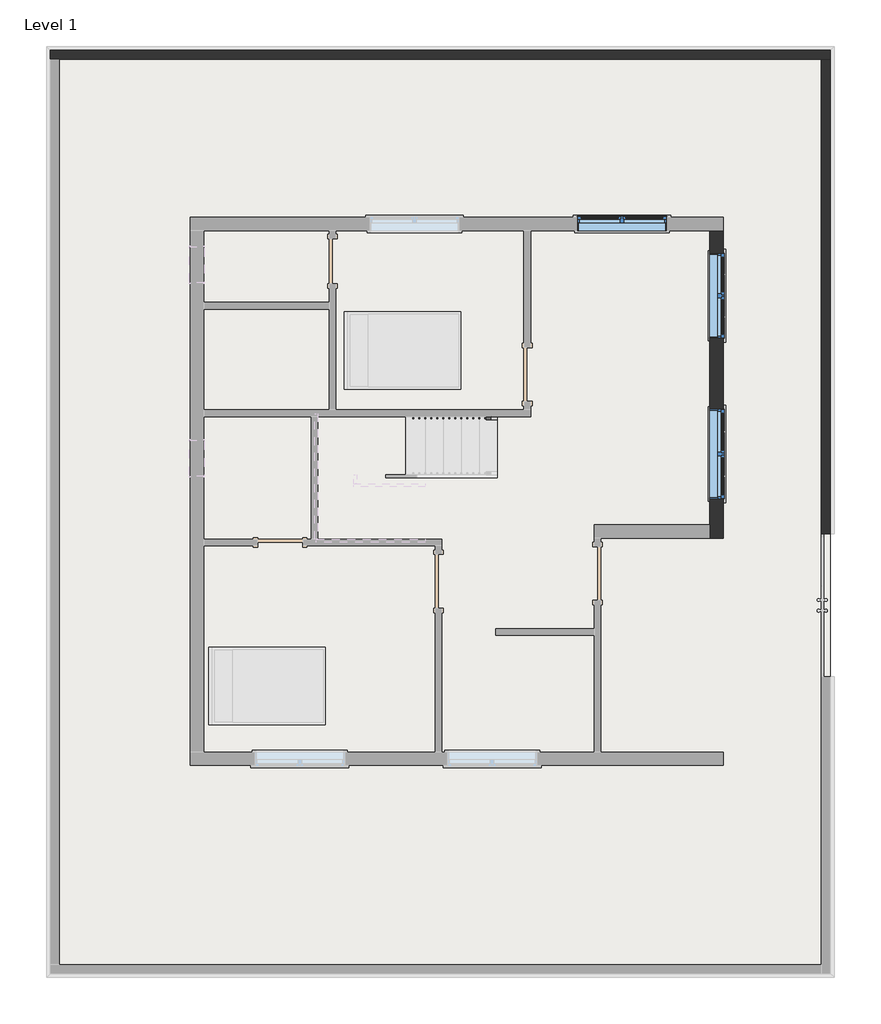
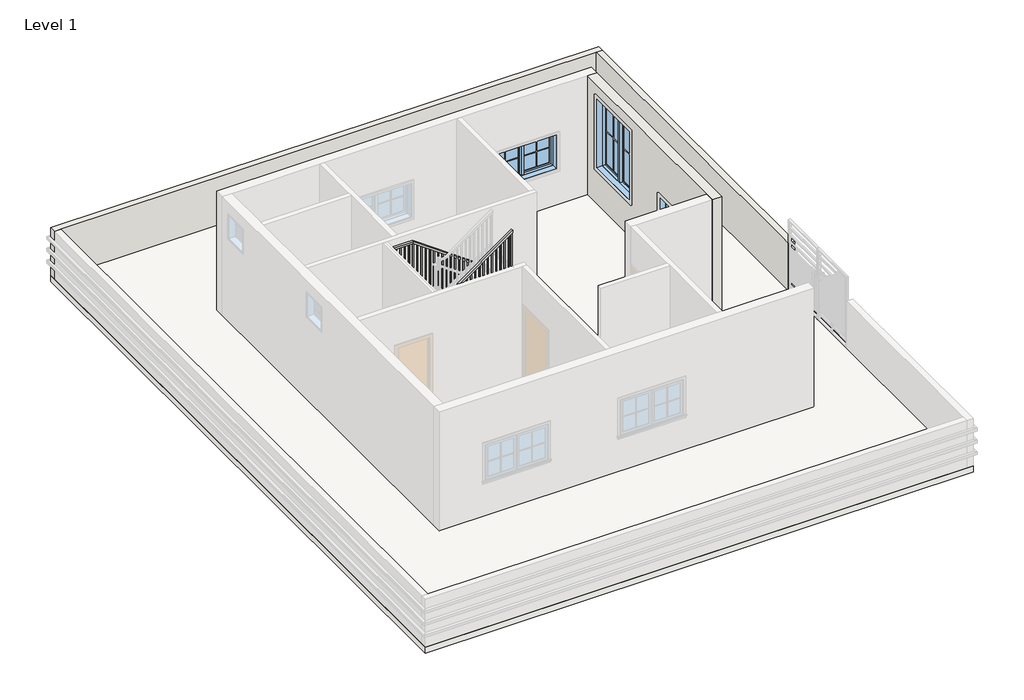
# One storey, part 2 of 3: 3 walls, 3 windows, 1 railing, 1 slab.
"""IFC4 building model written with IfcOpenShell, lengths in millimetres."""

from ifc_helpers import new_model, si_unit, frame, origin, place, context, project, spatial, polyline, outline, extrude, faceted_brep, transform, mapped, element, save
from components import window_9ac97e1a, window_c1d95f0f

model = new_model("IFC4")

# Units and contexts
model_context = context("Model", 3, world=origin())
ifc_project = project(units=[si_unit("LENGTHUNIT", "METRE", prefix="MILLI")], contexts=[model_context])

# Site, building, storey
site = spatial("IfcSite", under=ifc_project)
building = spatial("IfcBuilding", under=site)
storey = spatial("IfcBuildingStorey", under=building, Name="Level 1", Elevation=0.0)

# Railing
placement = place(None, origin())
element("IfcRailing", 1, ObjectType="Handrail - Rectangular", at=placement, inside=storey, context=model_context, shape_type="SolidModel", body=[
    faceted_brep([(-569.5630704, 606.5457979, 1132.1142857), (-569.5630704, 606.5457979, 1069.6859823), (-569.5630704, 657.3457979, 1069.6859823), (-569.5630704, 657.3457979, 1132.1142857), (-3007.9630704, 606.5457979, 2873.8285714), (-3024.2426952, 606.5457979, 2823.0285714), (-3024.2426952, 657.3457979, 2823.0285714), (-3007.9630704, 657.3457979, 2873.8285714), (-3566.7630704, 606.5457979, 2873.8285714), (-3566.7630704, 606.5457979, 2823.0285714), (-3617.5630704, 657.3457979, 2823.0285714), (-3617.5630704, 657.3457979, 2873.8285714), (-3566.7630704, -1374.6542021, 2873.8285714), (-3566.7630704, -1374.6542021, 2823.0285714), (-3617.5630704, -1425.4542021, 2823.0285714), (-3617.5630704, -1425.4542021, 2873.8285714), (-3312.7630704, -1374.6542021, 2873.8285714), (-3296.4834457, -1374.6542021, 2823.0285714), (-3296.4834457, -1425.4542021, 2823.0285714), (-3312.7630704, -1425.4542021, 2873.8285714), (-1788.7630704, -1374.6542021, 3962.4), (-1788.7630704, -1425.4542021, 3962.4), (-1788.7630704, -1425.4542021, 3899.9716966), (-1788.7630704, -1374.6542021, 3899.9716966)], [[[0, 1, 2, 3]], [[1, 0, 4, 5]], [[2, 1, 5, 6]], [[3, 2, 6, 7]], [[0, 3, 7, 4]], [[5, 4, 8, 9]], [[6, 5, 9, 10]], [[7, 6, 10, 11]], [[4, 7, 11, 8]], [[9, 8, 12, 13]], [[10, 9, 13, 14]], [[11, 10, 14, 15]], [[8, 11, 15, 12]], [[13, 12, 16, 17]], [[14, 13, 17, 18]], [[15, 14, 18, 19]], [[12, 15, 19, 16]], [[20, 21, 22, 23]], [[17, 16, 20, 23]], [[18, 17, 23, 22]], [[19, 18, 22, 21]], [[16, 19, 21, 20]]]),
    extrude(outline(polyline([(3852.3466966, -1855.4380704), (3838.7395538, -1874.4880704), (2830.2857143, -1874.4880704), (2830.2857143, -1855.4380704), (3852.3466966, -1855.4380704)])), frame((0.0, -1409.5792021, 0.0), z_axis=(0.0, 1.0, 0.0), x_axis=(0.0, 0.0, 1.0)), (0.0, 0.0, 1.0), 19.05),
    extrude(outline(polyline([(3779.7752681, -1957.0380704), (3766.1681252, -1976.0880704), (2830.2857143, -1976.0880704), (2830.2857143, -1957.0380704), (3779.7752681, -1957.0380704)])), frame((0.0, -1409.5792021, 0.0), z_axis=(0.0, 1.0, 0.0), x_axis=(0.0, 0.0, 1.0)), (0.0, 0.0, 1.0), 19.05),
    extrude(outline(polyline([(3707.2038395, -2058.6380704), (3693.5966966, -2077.6880704), (2830.2857143, -2077.6880704), (2830.2857143, -2058.6380704), (3707.2038395, -2058.6380704)])), frame((0.0, -1409.5792021, 0.0), z_axis=(0.0, 1.0, 0.0), x_axis=(0.0, 0.0, 1.0)), (0.0, 0.0, 1.0), 19.05),
    extrude(outline(polyline([(3634.6324109, -2160.2380704), (3621.0252681, -2179.2880704), (2612.5714286, -2179.2880704), (2612.5714286, -2160.2380704), (3634.6324109, -2160.2380704)])), frame((0.0, -1409.5792021, 0.0), z_axis=(0.0, 1.0, 0.0), x_axis=(0.0, 0.0, 1.0)), (0.0, 0.0, 1.0), 19.05),
    extrude(outline(polyline([(3562.0609823, -2261.8380704), (3548.4538395, -2280.8880704), (2612.5714286, -2280.8880704), (2612.5714286, -2261.8380704), (3562.0609823, -2261.8380704)])), frame((0.0, -1409.5792021, 0.0), z_axis=(0.0, 1.0, 0.0), x_axis=(0.0, 0.0, 1.0)), (0.0, 0.0, 1.0), 19.05),
    extrude(outline(polyline([(3489.4895538, -2363.4380704), (3475.8824109, -2382.4880704), (2612.5714286, -2382.4880704), (2612.5714286, -2363.4380704), (3489.4895538, -2363.4380704)])), frame((0.0, -1409.5792021, 0.0), z_axis=(0.0, 1.0, 0.0), x_axis=(0.0, 0.0, 1.0)), (0.0, 0.0, 1.0), 19.05),
    extrude(outline(polyline([(3416.9181252, -2465.0380704), (3403.3109823, -2484.0880704), (2394.8571429, -2484.0880704), (2394.8571429, -2465.0380704), (3416.9181252, -2465.0380704)])), frame((0.0, -1409.5792021, 0.0), z_axis=(0.0, 1.0, 0.0), x_axis=(0.0, 0.0, 1.0)), (0.0, 0.0, 1.0), 19.05),
    extrude(outline(polyline([(3344.3466966, -2566.6380704), (3330.7395538, -2585.6880704), (2394.8571429, -2585.6880704), (2394.8571429, -2566.6380704), (3344.3466966, -2566.6380704)])), frame((0.0, -1409.5792021, 0.0), z_axis=(0.0, 1.0, 0.0), x_axis=(0.0, 0.0, 1.0)), (0.0, 0.0, 1.0), 19.05),
    extrude(outline(polyline([(3271.7752681, -2668.2380704), (3258.1681252, -2687.2880704), (2394.8571429, -2687.2880704), (2394.8571429, -2668.2380704), (3271.7752681, -2668.2380704)])), frame((0.0, -1409.5792021, 0.0), z_axis=(0.0, 1.0, 0.0), x_axis=(0.0, 0.0, 1.0)), (0.0, 0.0, 1.0), 19.05),
    extrude(outline(polyline([(3199.2038395, -2769.8380704), (3185.5966966, -2788.8880704), (2177.1428571, -2788.8880704), (2177.1428571, -2769.8380704), (3199.2038395, -2769.8380704)])), frame((0.0, -1409.5792021, 0.0), z_axis=(0.0, 1.0, 0.0), x_axis=(0.0, 0.0, 1.0)), (0.0, 0.0, 1.0), 19.05),
    extrude(outline(polyline([(3126.6324109, -2871.4380704), (3113.0252681, -2890.4880704), (2177.1428571, -2890.4880704), (2177.1428571, -2871.4380704), (3126.6324109, -2871.4380704)])), frame((0.0, -1409.5792021, 0.0), z_axis=(0.0, 1.0, 0.0), x_axis=(0.0, 0.0, 1.0)), (0.0, 0.0, 1.0), 19.05),
    extrude(outline(polyline([(3054.0609823, -2973.0380704), (3040.4538395, -2992.0880704), (2177.1428571, -2992.0880704), (2177.1428571, -2973.0380704), (3054.0609823, -2973.0380704)])), frame((0.0, -1409.5792021, 0.0), z_axis=(0.0, 1.0, 0.0), x_axis=(0.0, 0.0, 1.0)), (0.0, 0.0, 1.0), 19.05),
    extrude(outline(polyline([(2981.4895538, -3074.6380704), (2967.8824109, -3093.6880704), (1959.4285714, -3093.6880704), (1959.4285714, -3074.6380704), (2981.4895538, -3074.6380704)])), frame((0.0, -1409.5792021, 0.0), z_axis=(0.0, 1.0, 0.0), x_axis=(0.0, 0.0, 1.0)), (0.0, 0.0, 1.0), 19.05),
    extrude(outline(polyline([(2908.9181252, -3176.2380704), (2895.3109823, -3195.2880704), (1959.4285714, -3195.2880704), (1959.4285714, -3176.2380704), (2908.9181252, -3176.2380704)])), frame((0.0, -1409.5792021, 0.0), z_axis=(0.0, 1.0, 0.0), x_axis=(0.0, 0.0, 1.0)), (0.0, 0.0, 1.0), 19.05),
    extrude(outline(polyline([(2836.3466966, -3277.8380704), (2822.7395538, -3296.8880704), (1959.4285714, -3296.8880704), (1959.4285714, -3277.8380704), (2836.3466966, -3277.8380704)])), frame((0.0, -1409.5792021, 0.0), z_axis=(0.0, 1.0, 0.0), x_axis=(0.0, 0.0, 1.0)), (0.0, 0.0, 1.0), 19.05),
    extrude(outline(polyline([(-3398.4880704, -1409.5792021), (-3398.4880704, -1390.5292021), (-3379.4380704, -1390.5292021), (-3379.4380704, -1409.5792021), (-3398.4880704, -1409.5792021)])), frame((0.0, 0.0, 1959.4285714), z_axis=(0.0, 0.0, 1.0), x_axis=(1.0, 0.0, 0.0)), (0.0, 0.0, 1.0), 863.6),
    extrude(outline(polyline([(-3500.0880704, -1409.5792021), (-3500.0880704, -1390.5292021), (-3481.0380704, -1390.5292021), (-3481.0380704, -1409.5792021), (-3500.0880704, -1409.5792021)])), frame((0.0, 0.0, 1959.4285714), z_axis=(0.0, 0.0, 1.0), x_axis=(1.0, 0.0, 0.0)), (0.0, 0.0, 1.0), 863.6),
    extrude(outline(polyline([(-3601.6880704, -1288.9292021), (-3582.6380704, -1288.9292021), (-3582.6380704, -1307.9792021), (-3601.6880704, -1307.9792021), (-3601.6880704, -1288.9292021)])), frame((0.0, 0.0, 1959.4285714), z_axis=(0.0, 0.0, 1.0), x_axis=(1.0, 0.0, 0.0)), (0.0, 0.0, 1.0), 863.6),
    extrude(outline(polyline([(-3601.6880704, -1187.3292021), (-3582.6380704, -1187.3292021), (-3582.6380704, -1206.3792021), (-3601.6880704, -1206.3792021), (-3601.6880704, -1187.3292021)])), frame((0.0, 0.0, 1959.4285714), z_axis=(0.0, 0.0, 1.0), x_axis=(1.0, 0.0, 0.0)), (0.0, 0.0, 1.0), 863.6),
    extrude(outline(polyline([(-3601.6880704, -1085.7292021), (-3582.6380704, -1085.7292021), (-3582.6380704, -1104.7792021), (-3601.6880704, -1104.7792021), (-3601.6880704, -1085.7292021)])), frame((0.0, 0.0, 1959.4285714), z_axis=(0.0, 0.0, 1.0), x_axis=(1.0, 0.0, 0.0)), (0.0, 0.0, 1.0), 863.6),
    extrude(outline(polyline([(-3601.6880704, -984.1292021), (-3582.6380704, -984.1292021), (-3582.6380704, -1003.1792021), (-3601.6880704, -1003.1792021), (-3601.6880704, -984.1292021)])), frame((0.0, 0.0, 1959.4285714), z_axis=(0.0, 0.0, 1.0), x_axis=(1.0, 0.0, 0.0)), (0.0, 0.0, 1.0), 863.6),
    extrude(outline(polyline([(-3601.6880704, -882.5292021), (-3582.6380704, -882.5292021), (-3582.6380704, -901.5792021), (-3601.6880704, -901.5792021), (-3601.6880704, -882.5292021)])), frame((0.0, 0.0, 1959.4285714), z_axis=(0.0, 0.0, 1.0), x_axis=(1.0, 0.0, 0.0)), (0.0, 0.0, 1.0), 863.6),
    extrude(outline(polyline([(-3601.6880704, -780.9292021), (-3582.6380704, -780.9292021), (-3582.6380704, -799.9792021), (-3601.6880704, -799.9792021), (-3601.6880704, -780.9292021)])), frame((0.0, 0.0, 1959.4285714), z_axis=(0.0, 0.0, 1.0), x_axis=(1.0, 0.0, 0.0)), (0.0, 0.0, 1.0), 863.6),
    extrude(outline(polyline([(-3601.6880704, -679.3292021), (-3582.6380704, -679.3292021), (-3582.6380704, -698.3792021), (-3601.6880704, -698.3792021), (-3601.6880704, -679.3292021)])), frame((0.0, 0.0, 1959.4285714), z_axis=(0.0, 0.0, 1.0), x_axis=(1.0, 0.0, 0.0)), (0.0, 0.0, 1.0), 863.6),
    extrude(outline(polyline([(-3601.6880704, -577.7292021), (-3582.6380704, -577.7292021), (-3582.6380704, -596.7792021), (-3601.6880704, -596.7792021), (-3601.6880704, -577.7292021)])), frame((0.0, 0.0, 1959.4285714), z_axis=(0.0, 0.0, 1.0), x_axis=(1.0, 0.0, 0.0)), (0.0, 0.0, 1.0), 863.6),
    extrude(outline(polyline([(-3601.6880704, -476.1292021), (-3582.6380704, -476.1292021), (-3582.6380704, -495.1792021), (-3601.6880704, -495.1792021), (-3601.6880704, -476.1292021)])), frame((0.0, 0.0, 1959.4285714), z_axis=(0.0, 0.0, 1.0), x_axis=(1.0, 0.0, 0.0)), (0.0, 0.0, 1.0), 863.6),
    extrude(outline(polyline([(-3601.6880704, -374.5292021), (-3582.6380704, -374.5292021), (-3582.6380704, -393.5792021), (-3601.6880704, -393.5792021), (-3601.6880704, -374.5292021)])), frame((0.0, 0.0, 1959.4285714), z_axis=(0.0, 0.0, 1.0), x_axis=(1.0, 0.0, 0.0)), (0.0, 0.0, 1.0), 863.6),
    extrude(outline(polyline([(-3601.6880704, -272.9292021), (-3582.6380704, -272.9292021), (-3582.6380704, -291.9792021), (-3601.6880704, -291.9792021), (-3601.6880704, -272.9292021)])), frame((0.0, 0.0, 1959.4285714), z_axis=(0.0, 0.0, 1.0), x_axis=(1.0, 0.0, 0.0)), (0.0, 0.0, 1.0), 863.6),
    extrude(outline(polyline([(-3601.6880704, -171.3292021), (-3582.6380704, -171.3292021), (-3582.6380704, -190.3792021), (-3601.6880704, -190.3792021), (-3601.6880704, -171.3292021)])), frame((0.0, 0.0, 1959.4285714), z_axis=(0.0, 0.0, 1.0), x_axis=(1.0, 0.0, 0.0)), (0.0, 0.0, 1.0), 863.6),
    extrude(outline(polyline([(-3601.6880704, -69.7292021), (-3582.6380704, -69.7292021), (-3582.6380704, -88.7792021), (-3601.6880704, -88.7792021), (-3601.6880704, -69.7292021)])), frame((0.0, 0.0, 1959.4285714), z_axis=(0.0, 0.0, 1.0), x_axis=(1.0, 0.0, 0.0)), (0.0, 0.0, 1.0), 863.6),
    extrude(outline(polyline([(-3601.6880704, 31.8707979), (-3582.6380704, 31.8707979), (-3582.6380704, 12.8207979), (-3601.6880704, 12.8207979), (-3601.6880704, 31.8707979)])), frame((0.0, 0.0, 1959.4285714), z_axis=(0.0, 0.0, 1.0), x_axis=(1.0, 0.0, 0.0)), (0.0, 0.0, 1.0), 863.6),
    extrude(outline(polyline([(-3601.6880704, 133.4707979), (-3582.6380704, 133.4707979), (-3582.6380704, 114.4207979), (-3601.6880704, 114.4207979), (-3601.6880704, 133.4707979)])), frame((0.0, 0.0, 1959.4285714), z_axis=(0.0, 0.0, 1.0), x_axis=(1.0, 0.0, 0.0)), (0.0, 0.0, 1.0), 863.6),
    extrude(outline(polyline([(-3601.6880704, 235.0707979), (-3582.6380704, 235.0707979), (-3582.6380704, 216.0207979), (-3601.6880704, 216.0207979), (-3601.6880704, 235.0707979)])), frame((0.0, 0.0, 1959.4285714), z_axis=(0.0, 0.0, 1.0), x_axis=(1.0, 0.0, 0.0)), (0.0, 0.0, 1.0), 863.6),
    extrude(outline(polyline([(-3601.6880704, 336.6707979), (-3582.6380704, 336.6707979), (-3582.6380704, 317.6207979), (-3601.6880704, 317.6207979), (-3601.6880704, 336.6707979)])), frame((0.0, 0.0, 1959.4285714), z_axis=(0.0, 0.0, 1.0), x_axis=(1.0, 0.0, 0.0)), (0.0, 0.0, 1.0), 863.6),
    extrude(outline(polyline([(-3601.6880704, 438.2707979), (-3582.6380704, 438.2707979), (-3582.6380704, 419.2207979), (-3601.6880704, 419.2207979), (-3601.6880704, 438.2707979)])), frame((0.0, 0.0, 1959.4285714), z_axis=(0.0, 0.0, 1.0), x_axis=(1.0, 0.0, 0.0)), (0.0, 0.0, 1.0), 863.6),
    extrude(outline(polyline([(-3601.6880704, 539.8707979), (-3582.6380704, 539.8707979), (-3582.6380704, 520.8207979), (-3601.6880704, 520.8207979), (-3601.6880704, 539.8707979)])), frame((0.0, 0.0, 1959.4285714), z_axis=(0.0, 0.0, 1.0), x_axis=(1.0, 0.0, 0.0)), (0.0, 0.0, 1.0), 863.6),
    extrude(outline(polyline([(-3506.4380704, 641.4707979), (-3506.4380704, 622.4207979), (-3525.4880704, 622.4207979), (-3525.4880704, 641.4707979), (-3506.4380704, 641.4707979)])), frame((0.0, 0.0, 1959.4285714), z_axis=(0.0, 0.0, 1.0), x_axis=(1.0, 0.0, 0.0)), (0.0, 0.0, 1.0), 863.6),
    extrude(outline(polyline([(-3404.8380704, 641.4707979), (-3404.8380704, 622.4207979), (-3423.8880704, 622.4207979), (-3423.8880704, 641.4707979), (-3404.8380704, 641.4707979)])), frame((0.0, 0.0, 1959.4285714), z_axis=(0.0, 0.0, 1.0), x_axis=(1.0, 0.0, 0.0)), (0.0, 0.0, 1.0), 863.6),
    extrude(outline(polyline([(-3303.2380704, 641.4707979), (-3303.2380704, 622.4207979), (-3322.2880704, 622.4207979), (-3322.2880704, 641.4707979), (-3303.2380704, 641.4707979)])), frame((0.0, 0.0, 1959.4285714), z_axis=(0.0, 0.0, 1.0), x_axis=(1.0, 0.0, 0.0)), (0.0, 0.0, 1.0), 863.6),
    extrude(outline(polyline([(-3201.6380704, 641.4707979), (-3201.6380704, 622.4207979), (-3220.6880704, 622.4207979), (-3220.6880704, 641.4707979), (-3201.6380704, 641.4707979)])), frame((0.0, 0.0, 1959.4285714), z_axis=(0.0, 0.0, 1.0), x_axis=(1.0, 0.0, 0.0)), (0.0, 0.0, 1.0), 863.6),
    extrude(outline(polyline([(-3100.0380704, 641.4707979), (-3100.0380704, 622.4207979), (-3119.0880704, 622.4207979), (-3119.0880704, 641.4707979), (-3100.0380704, 641.4707979)])), frame((0.0, 0.0, 1959.4285714), z_axis=(0.0, 0.0, 1.0), x_axis=(1.0, 0.0, 0.0)), (0.0, 0.0, 1.0), 863.6),
    extrude(outline(polyline([(2804.5966966, -2998.4380704), (2818.2038395, -3017.4880704), (1959.4285714, -3017.4880704), (1959.4285714, -2998.4380704), (2804.5966966, -2998.4380704)])), frame((0.0, 622.4207979, 0.0), z_axis=(0.0, 1.0, 0.0), x_axis=(0.0, 0.0, 1.0)), (0.0, 0.0, 1.0), 19.05),
    extrude(outline(polyline([(2732.0252681, -2896.8380704), (2745.6324109, -2915.8880704), (1741.7142857, -2915.8880704), (1741.7142857, -2896.8380704), (2732.0252681, -2896.8380704)])), frame((0.0, 622.4207979, 0.0), z_axis=(0.0, 1.0, 0.0), x_axis=(0.0, 0.0, 1.0)), (0.0, 0.0, 1.0), 19.05),
    extrude(outline(polyline([(2659.4538395, -2795.2380704), (2673.0609823, -2814.2880704), (1741.7142857, -2814.2880704), (1741.7142857, -2795.2380704), (2659.4538395, -2795.2380704)])), frame((0.0, 622.4207979, 0.0), z_axis=(0.0, 1.0, 0.0), x_axis=(0.0, 0.0, 1.0)), (0.0, 0.0, 1.0), 19.05),
    extrude(outline(polyline([(2586.8824109, -2693.6380704), (2600.4895538, -2712.6880704), (1741.7142857, -2712.6880704), (1741.7142857, -2693.6380704), (2586.8824109, -2693.6380704)])), frame((0.0, 622.4207979, 0.0), z_axis=(0.0, 1.0, 0.0), x_axis=(0.0, 0.0, 1.0)), (0.0, 0.0, 1.0), 19.05),
    extrude(outline(polyline([(2514.3109823, -2592.0380704), (2527.9181252, -2611.0880704), (1524.0, -2611.0880704), (1524.0, -2592.0380704), (2514.3109823, -2592.0380704)])), frame((0.0, 622.4207979, 0.0), z_axis=(0.0, 1.0, 0.0), x_axis=(0.0, 0.0, 1.0)), (0.0, 0.0, 1.0), 19.05),
    extrude(outline(polyline([(2441.7395538, -2490.4380704), (2455.3466966, -2509.4880704), (1524.0, -2509.4880704), (1524.0, -2490.4380704), (2441.7395538, -2490.4380704)])), frame((0.0, 622.4207979, 0.0), z_axis=(0.0, 1.0, 0.0), x_axis=(0.0, 0.0, 1.0)), (0.0, 0.0, 1.0), 19.05),
    extrude(outline(polyline([(2369.1681252, -2388.8380704), (2382.7752681, -2407.8880704), (1524.0, -2407.8880704), (1524.0, -2388.8380704), (2369.1681252, -2388.8380704)])), frame((0.0, 622.4207979, 0.0), z_axis=(0.0, 1.0, 0.0), x_axis=(0.0, 0.0, 1.0)), (0.0, 0.0, 1.0), 19.05),
    extrude(outline(polyline([(2296.5966966, -2287.2380704), (2310.2038395, -2306.2880704), (1306.2857143, -2306.2880704), (1306.2857143, -2287.2380704), (2296.5966966, -2287.2380704)])), frame((0.0, 622.4207979, 0.0), z_axis=(0.0, 1.0, 0.0), x_axis=(0.0, 0.0, 1.0)), (0.0, 0.0, 1.0), 19.05),
    extrude(outline(polyline([(2224.0252681, -2185.6380704), (2237.6324109, -2204.6880704), (1306.2857143, -2204.6880704), (1306.2857143, -2185.6380704), (2224.0252681, -2185.6380704)])), frame((0.0, 622.4207979, 0.0), z_axis=(0.0, 1.0, 0.0), x_axis=(0.0, 0.0, 1.0)), (0.0, 0.0, 1.0), 19.05),
    extrude(outline(polyline([(2151.4538395, -2084.0380704), (2165.0609823, -2103.0880704), (1306.2857143, -2103.0880704), (1306.2857143, -2084.0380704), (2151.4538395, -2084.0380704)])), frame((0.0, 622.4207979, 0.0), z_axis=(0.0, 1.0, 0.0), x_axis=(0.0, 0.0, 1.0)), (0.0, 0.0, 1.0), 19.05),
    extrude(outline(polyline([(2078.8824109, -1982.4380704), (2092.4895538, -2001.4880704), (1088.5714286, -2001.4880704), (1088.5714286, -1982.4380704), (2078.8824109, -1982.4380704)])), frame((0.0, 622.4207979, 0.0), z_axis=(0.0, 1.0, 0.0), x_axis=(0.0, 0.0, 1.0)), (0.0, 0.0, 1.0), 19.05),
    extrude(outline(polyline([(2006.3109823, -1880.8380704), (2019.9181252, -1899.8880704), (1088.5714286, -1899.8880704), (1088.5714286, -1880.8380704), (2006.3109823, -1880.8380704)])), frame((0.0, 622.4207979, 0.0), z_axis=(0.0, 1.0, 0.0), x_axis=(0.0, 0.0, 1.0)), (0.0, 0.0, 1.0), 19.05),
    extrude(outline(polyline([(1933.7395538, -1779.2380704), (1947.3466966, -1798.2880704), (1088.5714286, -1798.2880704), (1088.5714286, -1779.2380704), (1933.7395538, -1779.2380704)])), frame((0.0, 622.4207979, 0.0), z_axis=(0.0, 1.0, 0.0), x_axis=(0.0, 0.0, 1.0)), (0.0, 0.0, 1.0), 19.05),
    extrude(outline(polyline([(1861.1681252, -1677.6380704), (1874.7752681, -1696.6880704), (870.8571429, -1696.6880704), (870.8571429, -1677.6380704), (1861.1681252, -1677.6380704)])), frame((0.0, 622.4207979, 0.0), z_axis=(0.0, 1.0, 0.0), x_axis=(0.0, 0.0, 1.0)), (0.0, 0.0, 1.0), 19.05),
    extrude(outline(polyline([(1788.5966966, -1576.0380704), (1802.2038395, -1595.0880704), (870.8571429, -1595.0880704), (870.8571429, -1576.0380704), (1788.5966966, -1576.0380704)])), frame((0.0, 622.4207979, 0.0), z_axis=(0.0, 1.0, 0.0), x_axis=(0.0, 0.0, 1.0)), (0.0, 0.0, 1.0), 19.05),
    extrude(outline(polyline([(1716.0252681, -1474.4380704), (1729.6324109, -1493.4880704), (870.8571429, -1493.4880704), (870.8571429, -1474.4380704), (1716.0252681, -1474.4380704)])), frame((0.0, 622.4207979, 0.0), z_axis=(0.0, 1.0, 0.0), x_axis=(0.0, 0.0, 1.0)), (0.0, 0.0, 1.0), 19.05),
    extrude(outline(polyline([(1643.4538395, -1372.8380704), (1657.0609823, -1391.8880704), (653.1428571, -1391.8880704), (653.1428571, -1372.8380704), (1643.4538395, -1372.8380704)])), frame((0.0, 622.4207979, 0.0), z_axis=(0.0, 1.0, 0.0), x_axis=(0.0, 0.0, 1.0)), (0.0, 0.0, 1.0), 19.05),
    extrude(outline(polyline([(1570.8824109, -1271.2380704), (1584.4895538, -1290.2880704), (653.1428571, -1290.2880704), (653.1428571, -1271.2380704), (1570.8824109, -1271.2380704)])), frame((0.0, 622.4207979, 0.0), z_axis=(0.0, 1.0, 0.0), x_axis=(0.0, 0.0, 1.0)), (0.0, 0.0, 1.0), 19.05),
    extrude(outline(polyline([(1498.3109823, -1169.6380704), (1511.9181252, -1188.6880704), (653.1428571, -1188.6880704), (653.1428571, -1169.6380704), (1498.3109823, -1169.6380704)])), frame((0.0, 622.4207979, 0.0), z_axis=(0.0, 1.0, 0.0), x_axis=(0.0, 0.0, 1.0)), (0.0, 0.0, 1.0), 19.05),
    extrude(outline(polyline([(1425.7395538, -1068.0380704), (1439.3466966, -1087.0880704), (435.4285714, -1087.0880704), (435.4285714, -1068.0380704), (1425.7395538, -1068.0380704)])), frame((0.0, 622.4207979, 0.0), z_axis=(0.0, 1.0, 0.0), x_axis=(0.0, 0.0, 1.0)), (0.0, 0.0, 1.0), 19.05),
    extrude(outline(polyline([(1353.1681252, -966.4380704), (1366.7752681, -985.4880704), (435.4285714, -985.4880704), (435.4285714, -966.4380704), (1353.1681252, -966.4380704)])), frame((0.0, 622.4207979, 0.0), z_axis=(0.0, 1.0, 0.0), x_axis=(0.0, 0.0, 1.0)), (0.0, 0.0, 1.0), 19.05),
    extrude(outline(polyline([(1280.5966966, -864.8380704), (1294.2038395, -883.8880704), (435.4285714, -883.8880704), (435.4285714, -864.8380704), (1280.5966966, -864.8380704)])), frame((0.0, 622.4207979, 0.0), z_axis=(0.0, 1.0, 0.0), x_axis=(0.0, 0.0, 1.0)), (0.0, 0.0, 1.0), 19.05),
    extrude(outline(polyline([(1208.0252681, -763.2380704), (1221.6324109, -782.2880704), (217.7142857, -782.2880704), (217.7142857, -763.2380704), (1208.0252681, -763.2380704)])), frame((0.0, 622.4207979, 0.0), z_axis=(0.0, 1.0, 0.0), x_axis=(0.0, 0.0, 1.0)), (0.0, 0.0, 1.0), 19.05),
    extrude(outline(polyline([(1135.4538395, -661.6380704), (1149.0609823, -680.6880704), (217.7142857, -680.6880704), (217.7142857, -661.6380704), (1135.4538395, -661.6380704)])), frame((0.0, 622.4207979, 0.0), z_axis=(0.0, 1.0, 0.0), x_axis=(0.0, 0.0, 1.0)), (0.0, 0.0, 1.0), 19.05),
    extrude(outline(polyline([(-3601.6880704, -1390.5292021), (-3582.6380704, -1390.5292021), (-3582.6380704, -1409.5792021), (-3601.6880704, -1409.5792021), (-3601.6880704, -1390.5292021)])), frame((0.0, 0.0, 1959.4285714), z_axis=(0.0, 0.0, 1.0), x_axis=(1.0, 0.0, 0.0)), (0.0, 0.0, 1.0), 863.6),
    extrude(outline(polyline([(-3582.6380704, 641.4707979), (-3582.6380704, 622.4207979), (-3601.6880704, 622.4207979), (-3601.6880704, 641.4707979), (-3582.6380704, 641.4707979)])), frame((0.0, 0.0, 1959.4285714), z_axis=(0.0, 0.0, 1.0), x_axis=(1.0, 0.0, 0.0)), (0.0, 0.0, 1.0), 863.6),
    extrude(outline(polyline([(3899.9716966, -1788.7630704), (3886.3645538, -1807.8130704), (2830.2857143, -1807.8130704), (2830.2857143, -1788.7630704), (3899.9716966, -1788.7630704)])), frame((0.0, -1409.5792021, 0.0), z_axis=(0.0, 1.0, 0.0), x_axis=(0.0, 0.0, 1.0)), (0.0, 0.0, 1.0), 19.05),
    extrude(outline(polyline([(1069.6859823, -569.5630704), (1083.2931252, -588.6130704), (217.7142857, -588.6130704), (217.7142857, -569.5630704), (1069.6859823, -569.5630704)])), frame((0.0, 622.4207979, 0.0), z_axis=(0.0, 1.0, 0.0), x_axis=(0.0, 0.0, 1.0)), (0.0, 0.0, 1.0), 19.05),
])

# Slab
element("IfcSlab", 2, ObjectType="floor 6\"", at=placement, inside=storey, context=model_context, shape_type="SweptSolid", body=[
    extrude(outline(polyline([(5094.585534, 6885.5791885), (5094.585534, -8811.6208115), (-8164.214466, -8811.6208115), (-8164.214466, 6885.5791885), (5094.585534, 6885.5791885)])), frame((0.0, 0.0, -152.4), z_axis=(0.0, 0.0, 1.0), x_axis=(1.0, 0.0, 0.0)), (0.0, 0.0, 1.0), 152.4),
])

# Walls
element("IfcWall", 3, at=placement, inside=storey, context=model_context, shape_type="Brep", body=[
    faceted_brep([(-8164.214466, 6733.1791885, 0.0), (-8011.814466, 6733.1791885, 0.0), (4942.185534, 6733.1791885, 0.0), (5094.585534, 6733.1791885, 0.0), (5094.585534, 6733.1791885, 304.8), (5069.185534, 6733.1791885, 304.8), (5069.185534, 6733.1791885, 372.5333333), (5094.585534, 6733.1791885, 372.5333333), (5094.585534, 6733.1791885, 609.6), (5069.185534, 6733.1791885, 609.6), (5069.185534, 6733.1791885, 677.3333333), (5094.585534, 6733.1791885, 677.3333333), (5094.585534, 6733.1791885, 914.4), (5069.185534, 6733.1791885, 914.4), (5069.185534, 6733.1791885, 982.1333333), (5094.585534, 6733.1791885, 982.1333333), (5094.585534, 6733.1791885, 1219.2), (4942.185534, 6733.1791885, 1219.2), (-8011.814466, 6733.1791885, 1219.2), (-8164.214466, 6733.1791885, 1219.2), (-8164.214466, 6733.1791885, 982.1333333), (-8138.814466, 6733.1791885, 982.1333333), (-8138.814466, 6733.1791885, 914.4), (-8164.214466, 6733.1791885, 914.4), (-8164.214466, 6733.1791885, 677.3333333), (-8138.814466, 6733.1791885, 677.3333333), (-8138.814466, 6733.1791885, 609.6), (-8164.214466, 6733.1791885, 609.6), (-8164.214466, 6733.1791885, 372.5333333), (-8138.814466, 6733.1791885, 372.5333333), (-8138.814466, 6733.1791885, 304.8), (-8164.214466, 6733.1791885, 304.8), (5094.585534, 6885.5791885, 0.0), (-8164.214466, 6885.5791885, 0.0), (-8164.214466, 6885.5791885, 304.8), (5094.585534, 6885.5791885, 304.8), (-8164.214466, 6885.5791885, 1219.2), (5094.585534, 6885.5791885, 1219.2), (5094.585534, 6885.5791885, 982.1333333), (-8164.214466, 6885.5791885, 982.1333333), (5094.585534, 6885.5791885, 372.5333333), (-8164.214466, 6885.5791885, 372.5333333), (-8164.214466, 6885.5791885, 609.6), (5094.585534, 6885.5791885, 609.6), (5094.585534, 6885.5791885, 677.3333333), (-8164.214466, 6885.5791885, 677.3333333), (-8164.214466, 6885.5791885, 914.4), (5094.585534, 6885.5791885, 914.4), (-8138.814466, 6860.1791885, 304.8), (-8138.814466, 6860.1791885, 372.5333333), (5069.185534, 6860.1791885, 372.5333333), (5069.185534, 6860.1791885, 304.8), (5069.185534, 6860.1791885, 677.3333333), (-8138.814466, 6860.1791885, 677.3333333), (-8138.814466, 6860.1791885, 609.6), (5069.185534, 6860.1791885, 609.6), (5069.185534, 6860.1791885, 982.1333333), (-8138.814466, 6860.1791885, 982.1333333), (-8138.814466, 6860.1791885, 914.4), (5069.185534, 6860.1791885, 914.4)], [[[0, 1, 2, 3, 4, 5, 6, 7, 8, 9, 10, 11, 12, 13, 14, 15, 16, 17, 18, 19, 20, 21, 22, 23, 24, 25, 26, 27, 28, 29, 30, 31]], [[32, 33, 34, 35]], [[36, 37, 38, 39]], [[40, 41, 42, 43]], [[44, 45, 46, 47]], [[3, 2, 1, 0, 33, 32]], [[19, 18, 17, 16, 37, 36]], [[3, 32, 35, 4]], [[37, 16, 15, 38]], [[7, 40, 43, 8]], [[11, 44, 47, 12]], [[19, 36, 39, 20]], [[33, 0, 31, 34]], [[41, 28, 27, 42]], [[45, 24, 23, 46]], [[48, 49, 50, 51]], [[51, 50, 6, 5]], [[50, 49, 29, 28, 41, 40, 7, 6]], [[48, 51, 5, 4, 35, 34, 31, 30]], [[49, 48, 30, 29]], [[52, 53, 25, 24, 45, 44, 11, 10]], [[54, 55, 9, 8, 43, 42, 27, 26]], [[53, 54, 26, 25]], [[53, 52, 55, 54]], [[55, 52, 10, 9]], [[56, 57, 21, 20, 39, 38, 15, 14]], [[58, 59, 13, 12, 47, 46, 23, 22]], [[57, 58, 22, 21]], [[57, 56, 59, 58]], [[59, 56, 14, 13]]]),
])
element("IfcWall", 4, at=placement, inside=storey, context=model_context, shape_type="SweptSolid", body=[
    extrude(outline(polyline([(1219.2, 4942.185534), (0.0, 4942.185534), (0.0, 5094.585534), (304.8, 5094.585534), (304.8, 5069.185534), (372.5333333, 5069.185534), (372.5333333, 5094.585534), (609.6, 5094.585534), (609.6, 5069.185534), (677.3333333, 5069.185534), (677.3333333, 5094.585534), (914.4, 5094.585534), (914.4, 5069.185534), (982.1333333, 5069.185534), (982.1333333, 5094.585534), (1219.2, 5094.585534), (1219.2, 4942.185534)])), frame((0.0, -1330.2042021, 0.0), z_axis=(0.0, 1.0, 0.0), x_axis=(0.0, 0.0, 1.0)), (0.0, 0.0, 1.0), 8063.3833906),
])
element("IfcWall", 5, ObjectType="WALL 9\"", at=placement, inside=storey, context=model_context, shape_type="Brep", body=[
    faceted_brep([(3049.9369296, 3819.6457979, 0.0), (3049.9369296, -1184.1542021, 0.0), (3049.9369296, -1412.7542021, 0.0), (3049.9369296, -1412.7542021, 355.6), (3049.9369296, -1412.7542021, 423.3333333), (3049.9369296, -1412.7542021, 3048.0), (3049.9369296, -1184.1542021, 3048.0), (3049.9369296, 3819.6457979, 3048.0), (3049.9369296, -739.6542021, 1828.8), (3049.9369296, -739.6542021, 914.4), (3049.9369296, 784.3457979, 914.4), (3049.9369296, 784.3457979, 1828.8), (3049.9369296, 1990.8457979, 2743.2), (3049.9369296, 1990.8457979, 914.4), (3049.9369296, 3438.6457979, 914.4), (3049.9369296, 3438.6457979, 2743.2), (3278.5369296, 3819.6457979, 0.0), (3278.5369296, 3819.6457979, 355.6), (3278.5369296, 3819.6457979, 423.3333333), (3278.5369296, 3819.6457979, 3048.0), (3278.5369296, -1412.7542021, 3048.0), (3278.5369296, -1412.7542021, 0.0), (3278.5369296, -739.6542021, 1828.8), (3278.5369296, 784.3457979, 1828.8), (3278.5369296, 784.3457979, 914.4), (3278.5369296, -739.6542021, 914.4), (3278.5369296, 1990.8457979, 2743.2), (3278.5369296, 3438.6457979, 2743.2), (3278.5369296, 3438.6457979, 914.4), (3278.5369296, 1990.8457979, 914.4)], [[[0, 1, 2, 3, 4, 5, 6, 7], [8, 9, 10, 11], [12, 13, 14, 15]], [[16, 17, 18, 19, 20, 21], [22, 23, 24, 25], [26, 27, 28, 29]], [[2, 1, 0, 16, 21]], [[0, 7, 19, 18, 17, 16]], [[5, 4, 3, 2, 21, 20]], [[9, 8, 22, 25]], [[10, 9, 25, 24]], [[11, 10, 24, 23]], [[8, 11, 23, 22]], [[13, 12, 26, 29]], [[14, 13, 29, 28]], [[15, 14, 28, 27]], [[12, 15, 27, 26]], [[7, 6, 5, 20, 19]]]),
])

# Windows
window_shape = window_9ac97e1a(model_context)
element("IfcWindow", 6, ObjectType="Window-Casement-Double : 57\" x 72\"", at=placement, inside=storey, context=model_context, shape_type="MappedRepresentation", body=[
    mapped(window_shape, transform((3164.2369296, 2714.7457979, 0.0), x_axis=(0.0, -1.0, 0.0), y_axis=(1.0, 0.0, 0.0), z_axis=(0.0, 0.0, 1.0))),
])
window_2_shape = window_c1d95f0f(model_context)
element("IfcWindow", 7, ObjectType="Window-Casement-Double : WINDOW 6\"", at=placement, inside=storey, context=model_context, shape_type="MappedRepresentation", body=[
    mapped(window_2_shape, transform((3164.2369296, 22.3457979, 0.0), x_axis=(0.0, -1.0, 0.0), y_axis=(1.0, 0.0, 0.0), z_axis=(0.0, 0.0, 1.0))),
])
element("IfcWindow", 8, ObjectType="Window-Casement-Double : WINDOW 6\"", at=placement, inside=storey, context=model_context, shape_type="MappedRepresentation", body=[
    mapped(window_2_shape, transform((1554.5119296, 3933.9457979, 0.0), x_axis=(1.0, 0.0, 0.0), y_axis=(0.0, 1.0, 0.0), z_axis=(0.0, 0.0, 1.0))),
])

save(model, "model.ifc")

# Revit data of these elements
# Type "Handrail - Rectangular"
#   Assembly Code = "C2010400"
#   built-in parameter 1008612 = 0.0416667 (stored number, unit not read)
#   built-in parameter 1008611 = 0.0416667 (stored number, unit not read)
#   built-in parameter 1008609 = 0.333333 (stored number, unit not read)
#   built-in parameter 1008604 = 0.166667 (stored number, unit not read)
#   built-in parameter 1008603 = 0.166667 (stored number, unit not read)
#   Railing Height = 3' - 0"
#   built-in parameter 1008630 = 2
#   built-in parameter 1008610 = 2
#   built-in parameter 1008618 = Baluster - Square : 3/4"
# Type "floor 6\""
#   Assembly Code = "B1010"
#   Function = 0
#   Layers, outside or top first: 0' - 6" no material (function 1)
# Type
#   Assembly Code = "B2010"
#   Layers, outside or top first: 0' - 6" "Brick, Soldier Course" (function 1)
# Type "WALL 9\""
#   Assembly Code = "B2010"
#   Layers, outside or top first: 0' - 9" no material (function 1)
# Type "Window-Casement-Double : 57\" x 72\""
#   Type Mark = "17"
#   Fire Rating = "0.5h"
#   Assembly Code = "B2020100"
#   Analytic Construction = "Double glazing - domestic"
#   Frame Extension [instance default] = 0' - 0 1/4"
#   Window Inset [instance default] = 0' - 0"
#   Wall Thickness [instance default] = 0' - 6"
#   Interior Wall Closure [instance default] = 0' - 2 1/4"
#   Half Width = 2' - 4 1/2"
#   Visual Light Transmittance = 0.81
#   Thermal Resistance (R) = 1.8146 (h·ft²·°F)/BTU
#   Solar Heat Gain Coefficient = 0.76
#   Rough Width = 4' - 9 1/2"
#   Rough Height = 6' - 0 1/2"
#   Height = 6' - 0"
#   Heat Transfer Coefficient (U) = 0.5511 BTU/(h·ft²·°F)
#   Exterior Wall Closure [instance default] = 0' - 1 1/4"
#   Extension Jamb [instance default] = 0' - 2 1/4"
#   Default Sill Height = 3' - 0"
#   Width = 4' - 9"
#   Define Thermal Properties by = 0
#   Muntin Visibility = yes
#   Interior Trim Visibility [instance default] = yes
#   Exterior Trim Visibility [instance default] = yes
#   Extension Jamb Visibility [instance default] = yes
#   Interior Trim Material = Wood - Stained
#   Muntin Pattern = Muntin Pattern_2x2 : Muntin Pattern_2x2
#   Interior Trim = Trim-Window-Interior-Flat : Picture Frame
#   Interior Frame Material = Wood - Stained
#   Glass Panel Material = Glass
#   Exterior Trim Material = Clad - White
#   Exterior Trim = Trim-Window-Exterior-Flat : with Sill
#   Exterior Frame Material = Clad - White
#   Wall Closure = (empty or 0)
# Type "Window-Casement-Double : WINDOW 6\""
#   Type Mark = "18"
#   Fire Rating = "0.5h"
#   Assembly Code = "B2020100"
#   Analytic Construction = "Double glazing - domestic"
#   Frame Extension [instance default] = 0' - 0 1/4"
#   Window Inset [instance default] = 0' - 0"
#   Wall Thickness [instance default] = 0' - 6"
#   Interior Wall Closure [instance default] = 0' - 2 1/4"
#   Half Width = 2' - 6"
#   Visual Light Transmittance = 0.81
#   Thermal Resistance (R) = 1.8146 (h·ft²·°F)/BTU
#   Solar Heat Gain Coefficient = 0.76
#   Rough Width = 5' - 0 1/2"
#   Rough Height = 3' - 0 1/2"
#   Height = 3' - 0"
#   Heat Transfer Coefficient (U) = 0.5511 BTU/(h·ft²·°F)
#   Exterior Wall Closure [instance default] = 0' - 1 1/4"
#   Extension Jamb [instance default] = 0' - 2 1/4"
#   Default Sill Height = 3' - 0"
#   Width = 5' - 0"
#   Muntin Visibility = yes
#   Interior Trim Visibility [instance default] = yes
#   Exterior Trim Visibility [instance default] = yes
#   Extension Jamb Visibility [instance default] = yes
#   Interior Trim Material = Wood - Stained
#   Muntin Pattern = Muntin Pattern_2x2 : Muntin Pattern_2x2
#   Interior Trim = Trim-Window-Interior-Flat : Picture Frame
#   Interior Frame Material = Wood - Stained
#   Glass Panel Material = Glass
#   Exterior Trim Material = Clad - White
#   Exterior Trim = Trim-Window-Exterior-Flat : with Sill
#   Exterior Frame Material = Clad - White
#   Wall Closure = (empty or 0)
# Element 1 (IfcRailing, "Handrail - Rectangular")
#   Phase Created = New Construction
# Element 2 (IfcSlab, "floor 6\"")
#   Height Offset From Level = 0' - 0"
#   Phase Created = New Construction
#   Materials on its faces: "Clad - White", "Default Floor"
# Elements 3, 4 (IfcWall)
#   Top Offset = 0' - 0"
#   Base Offset = 0' - 0"
#   Unconnected Height = 4' - 0"
#   wall height = 4' - 0"
#   Phase Created = New Construction
#   Base Constraint = Level 1
#   Materials on its faces: "Brick, Soldier Course", "Parking Stripe", "Clad - White"
# Element 5 (IfcWall, "WALL 9\"")
#   Top Offset = 0' - 0"
#   Base Offset = 0' - 0"
#   Unconnected Height = 10' - 0"
#   wall height = 10' - 0"
#   Phase Created = New Construction
#   Base Constraint = Level 1
#   Materials on its faces: "Default Wall", "Wood - Stained"
# Element 6 (IfcWindow, "Window-Casement-Double : 57\" x 72\"")
#   Mark = "8"
#   Window Inset = 0' - 0"
#   Interior Wall Closure = 0' - 2 1/4"
#   Frame Extension = 0' - 0 1/4"
#   Exterior Wall Closure = 0' - 1 1/4"
#   Interior Trim Visibility = yes
#   Exterior Trim Visibility = yes
#   Phase Created = New Construction
#   Materials on its faces: "Wood - Stained", "Glass", "Clad - White"
# Element 7 (IfcWindow, "Window-Casement-Double : WINDOW 6\"")
#   Mark = "3"
#   Window Inset = 0' - 0"
#   Interior Wall Closure = 0' - 2 1/4"
#   Frame Extension = 0' - 0 1/4"
#   Exterior Wall Closure = 0' - 1 1/4"
#   Interior Trim Visibility = yes
#   Exterior Trim Visibility = yes
#   Phase Created = New Construction
#   Materials on its faces: "Wood - Stained", "Glass", "Clad - White"
# Element 8 (IfcWindow, "Window-Casement-Double : WINDOW 6\"")
#   Mark = "4"
#   Window Inset = 0' - 0"
#   Interior Wall Closure = 0' - 2 1/4"
#   Frame Extension = 0' - 0 1/4"
#   Exterior Wall Closure = 0' - 1 1/4"
#   Interior Trim Visibility = yes
#   Exterior Trim Visibility = yes
#   Phase Created = New Construction
#   Materials on its faces: "Wood - Stained", "Glass", "Clad - White"
# Materials
#   "Brick, Soldier Course": class "Masonry", colour RGB 170 98 104, transparency 0, Description = "Common brick soldier coursed", Cost = 0
#   "Wood - Stained": class "Wood", colour RGB 224 178 126, transparency 0, Cost = 0
#   "Glass": class "Glass", colour RGB 0 128 192, transparency 0.75, Description = "Soda Lime Glass", Cost = 0
#   "Clad - White": class "Wood", colour RGB 242 242 238, transparency 0, Cost = 0
#   "Default Floor": colour RGB 128 128 128, transparency 0, Cost = 0
#   "Parking Stripe": class "Paint", colour RGB 250 250 91, transparency 0, Cost = 0
#   "Default Wall": colour RGB 128 128 128, transparency 0, Cost = 0
